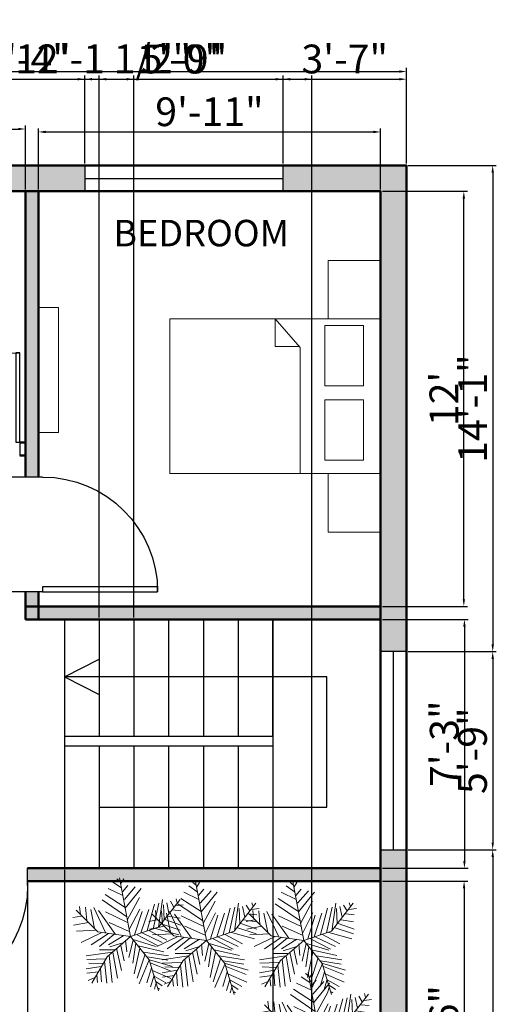
# Model space of a CAD drawing. Units: inches. Extents: x 1344 to 2521, y 3236 to 4924.
# Tile 7 of 14: x 2244 to 2410, y 3472 to 3814. Entities that reach past the tile are written whole.
import ezdxf

# ---------------------------------------------------------------- set-up
doc = ezdxf.new("R2010")
doc.units = ezdxf.units.IN
for name, color, linetype, lineweight in [('A-ANNO-DIMS', 2, 'Continuous', 18), ('A-AREA-IDEN', 3, 'Continuous', 18), ('A-DOOR', 50, 'Continuous', 25), ('A-FLOR-STRS', 7, 'Continuous', 25), ('A-FURN', 130, 'Continuous', 18), ('A-GLAZ', 150, 'Continuous', 25), ('A-WALL', 31, 'Continuous', 50), ('A-WALL-PATT', 8, 'Continuous', 13), ('L-PLNT', 82, 'Continuous', 13)]:
    doc.layers.add(name, color=color, linetype=linetype, lineweight=lineweight)
doc.styles.get("Standard").update_dxf_attribs({"font": 'arial.ttf'})
doc.dimstyles.new('ISO-25', dxfattribs={"dimtxt": 10, "dimasz": 2.5, "dimexe": 1.25, "dimexo": 0.625, "dimtad": 1, "dimdec": 0, "dimlunit": 4, "dimtxsty": 'Standard', "dimcen": 2.5, "dimadec": 0, "dimazin": 0, "dimtfac": 1, "dimtdec": 0, "dimtmove": 0, "dimatfit": 3, "dimfxl": 1, "dimarcsym": 0})

# ---------------------------------------------------------------- blocks, each defined once
blk = doc.blocks.new('*U2')
for p, q in [((0, 0), (0, -6)), ((40, 0), (40, -6))]:
    blk.add_line(p, q)
blk.add_lwpolyline([(0, 0), (0, 40), (1.75, 40), (1.75, 0)], close=True)
blk.add_arc((0, 0), 40, 0, 90)
blk = doc.blocks.new('*U8')
for p, q in [((-8.737, 47.138), (-17.069, 52.711)), ((-10.186, 53.64), (-13.084, 55.962)), ((0, 0), (-10.5, 57)), ((-9.099, 51.782), (-6.563, 55.962)), ((-7.65, 43.423), (-2.578, 49.46)), ((-5.839, 35.992), (4.667, 48.067)), ((-5.114, 28.097), (-24.676, 40.636)), ((-7.288, 39.707), (-21.778, 46.673)), ((-5.114, 27.632), (10.463, 46.673)), ((-48.585, 21.131), (-49.309, 29.026)), ((-3.665, 19.273), (-27.574, 35.527)), ((-2.941, 16.486), (8.652, 37.85)), ((16.259, 5.805), (23.142, 31.348)), ((22.055, 7.198), (27.489, 32.277)), ((27, 9), (48, 36)), ((27.127, 9.056), (31.112, 35.992)), ((31.836, 30.883), (32.561, 16.486)), ((35.096, 32.741), (37.27, 22.524)), ((38.719, 34.134), (41.979, 28.561)), ((43.791, 29.954), (51.036, 30.883)), ((44.153, 36.456), (45.239, 32.741)), ((-47.498, 19.737), (-55.83, 18.344)), ((-31.5, 4.5), (-52.5, 25.5)), ((-43.513, 28.561), (-42.427, 15.558)), ((-38.442, 26.239), (-34.819, 7.663)), ((-35.544, 28.097), (-24.314, 3.947)), ((-14.533, 2.09), (-30.834, 25.31)), ((-24.314, 23.917), (-2.941, 13.7)), ((-1.129, 6.734), (9.014, 26.704)), ((3.942, 1.625), (11.187, 24.381)), ((10.101, 3.483), (17.708, 26.239)), ((36.183, 19.737), (48.137, 17.88)), ((40.53, 25.775), (48.862, 24.846)), ((-40.615, 13.7), (-55.105, 10.913)), ((-20.691, 13.7), (-1.129, 4.876)), ((29.662, 12.307), (48.137, 6.269)), ((33.285, 16.486), (48.862, 10.913)), ((-33.37, 6.269), (-52.207, 5.34)), ((-28.299, 3.483), (-47.86, -5.805)), ((-21.416, 3.018), (-38.079, -8.128)), ((0, 0), (-31.5, 4.5)), ((-15.982, 2.09), (-30.11, -9.521)), ((0, 0), (-22.5, -19.5)), ((-6.563, 1.161), (-21.416, -8.128)), ((0, 0), (27, 9)), ((0, 0), (18, -22.5)), ((6.478, 1.625), (26.04, -8.592)), ((11.187, 3.483), (30.749, -5.805)), ((18.07, 5.805), (35.096, -3.483)), ((24.229, 7.663), (46.688, 1.625)), ((-6.563, -5.805), (-19.967, -9.985)), ((-9.461, -8.592), (-6.201, -23.453)), ((-4.752, -3.483), (-3.665, -14.629)), ((2.493, -3.019), (-1.491, -20.202)), ((1.769, -2.555), (24.229, -9.521)), ((5.029, -6.27), (2.131, -25.775)), ((7.565, -9.056), (32.198, -14.629)), ((-17.431, -15.094), (-42.789, -18.809)), ((-15.257, -12.772), (-30.11, -12.772)), ((-20.691, -18.345), (-17.793, -44.352)), ((-17.069, -15.094), (-12.721, -40.172)), ((-13.446, -11.378), (-8.737, -32.741)), ((9.014, -11.378), (3.58, -35.992)), ((14.085, -16.951), (6.478, -40.172)), ((12.274, -15.094), (36.907, -18.809)), ((-24.314, -21.596), (-42.427, -22.06)), ((-26.849, -26.24), (-40.253, -25.775)), ((-22.5, -19.5), (-37.5, -45)), ((-25.038, -23.918), (-22.865, -45.281)), ((18.07, -22.524), (8.289, -45.745)), ((16.259, -19.738), (36.183, -22.989)), ((18, -22.5), (27, -52.5)), ((18.433, -22.524), (40.53, -29.026)), ((19.157, -25.311), (38.719, -33.206)), ((-28.299, -29.026), (-42.789, -31.348)), ((-30.834, -34.135), (-42.427, -35.528)), ((-32.646, -36.921), (-31.921, -44.352)), ((-29.023, -30.884), (-27.936, -43.887)), ((20.244, -30.419), (15.897, -44.816)), ((22.78, -37.85), (19.519, -48.532)), ((21.331, -32.741), (39.081, -40.636)), ((-34.457, -39.708), (-40.978, -42.494)), ((22.78, -38.314), (34.372, -44.816)), ((24.591, -45.745), (23.142, -50.854)), ((24.591, -43.423), (30.749, -47.603)), ((26.764, -49.925), (28.213, -50.854))]:
    blk.add_line(p, q)
blk = doc.blocks.new('*D47')
at = {"layer": 'A-ANNO-DIMS', "color": 0, "lineweight": -2, "transparency": 16777216}
for p, q in [((2018.36, 3764.06), (2018.36, 3797.35)), ((2020.86, 3796.1), (2375.86, 3796.1)), ((2378.36, 3764.06), (2378.36, 3797.35))]:
    blk.add_line(p, q, dxfattribs=at)
at = {"layer": 'A-ANNO-DIMS', "color": 0, "lineweight": 100, "transparency": 16777216}
for points in [[(2020.86, 3796.52), (2020.86, 3795.69), (2018.36, 3796.1)], [(2375.86, 3796.52), (2375.86, 3795.69), (2378.36, 3796.1)]]:
    blk.add_solid(points, dxfattribs=at)
at = {"layer": 'Defpoints', "color": 0, "lineweight": 100, "transparency": 16777216}
for p in [(2378.36, 3796.1), (2018.36, 3763.43), (2378.36, 3763.43)]:
    blk.add_point(p, dxfattribs=at)
at = {"layer": 'A-ANNO-DIMS', "color": 0, "transparency": 16777216, "insert": (2198.36, 3801.84), "char_height": 10, "attachment_point": 5}
blk.add_mtext("30'", dxfattribs=at)
blk = doc.blocks.new('*D49')
at = {"layer": 'A-ANNO-DIMS', "color": 0, "lineweight": -2, "transparency": 16777216}
for p, q in [((2176.1, 3755.06), (2176.1, 3777.36)), ((2178.6, 3776.11), (2243.29, 3776.11)), ((2245.79, 3755.06), (2245.79, 3777.36))]:
    blk.add_line(p, q, dxfattribs=at)
at = {"layer": 'A-ANNO-DIMS', "color": 0, "lineweight": 100, "transparency": 16777216}
for points in [[(2178.6, 3776.53), (2178.6, 3775.69), (2176.1, 3776.11)], [(2243.29, 3776.53), (2243.29, 3775.69), (2245.79, 3776.11)]]:
    blk.add_solid(points, dxfattribs=at)
at = {"layer": 'Defpoints', "color": 0, "lineweight": 100, "transparency": 16777216}
for p in [(2245.79, 3776.11), (2176.1, 3754.43), (2245.79, 3754.43)]:
    blk.add_point(p, dxfattribs=at)
at = {"layer": 'A-ANNO-DIMS', "color": 0, "transparency": 16777216, "insert": (2210.94, 3781.84), "char_height": 10, "attachment_point": 5}
blk.add_mtext('5\'-10"', dxfattribs=at)
blk = doc.blocks.new('*D50')
at = {"layer": 'A-ANNO-DIMS', "color": 0, "lineweight": -2, "transparency": 16777216}
for p, q in [((2250.29, 3755.06), (2250.29, 3776.34)), ((2252.79, 3775.09), (2366.86, 3775.09)), ((2369.36, 3755.06), (2369.36, 3776.34))]:
    blk.add_line(p, q, dxfattribs=at)
at = {"layer": 'A-ANNO-DIMS', "color": 0, "lineweight": 100, "transparency": 16777216}
for points in [[(2252.79, 3775.5), (2252.79, 3774.67), (2250.29, 3775.09)], [(2366.86, 3775.5), (2366.86, 3774.67), (2369.36, 3775.09)]]:
    blk.add_solid(points, dxfattribs=at)
at = {"layer": 'Defpoints', "color": 0, "lineweight": 100, "transparency": 16777216}
for p in [(2369.36, 3775.09), (2250.29, 3754.43), (2369.36, 3754.43)]:
    blk.add_point(p, dxfattribs=at)
at = {"layer": 'A-ANNO-DIMS', "color": 0, "transparency": 16777216, "insert": (2309.83, 3780.82), "char_height": 10, "attachment_point": 5}
blk.add_mtext('9\'-11"', dxfattribs=at)
blk = doc.blocks.new('*D57')
at = {"layer": 'A-ANNO-DIMS', "color": 0, "lineweight": -2, "transparency": 16777216}
for p, q in [((2369.99, 3754.43), (2399.57, 3754.43)), ((2398.32, 3612.52), (2398.32, 3751.93)), ((2369.99, 3610.02), (2399.57, 3610.02))]:
    blk.add_line(p, q, dxfattribs=at)
at = {"layer": 'A-ANNO-DIMS', "color": 0, "lineweight": 100, "transparency": 16777216}
for points in [[(2397.9, 3751.93), (2398.73, 3751.93), (2398.32, 3754.43)], [(2397.9, 3612.52), (2398.73, 3612.52), (2398.32, 3610.02)]]:
    blk.add_solid(points, dxfattribs=at)
at = {"layer": 'Defpoints', "color": 0, "lineweight": 100, "transparency": 16777216}
for p in [(2369.36, 3754.43), (2398.32, 3754.43), (2369.36, 3610.02)]:
    blk.add_point(p, dxfattribs=at)
at = {"layer": 'A-ANNO-DIMS', "color": 0, "transparency": 16777216, "insert": (2392.67, 3682.23), "char_height": 10, "attachment_point": 5, "rotation": 90}
blk.add_mtext("12'", dxfattribs=at)
blk = doc.blocks.new('*D58')
at = {"layer": 'A-ANNO-DIMS', "color": 0, "lineweight": -2, "transparency": 16777216}
for p, q in [((2369.99, 3605.52), (2399.77, 3605.52)), ((2398.52, 3603.02), (2398.52, 3521.45)), ((2369.99, 3518.95), (2399.77, 3518.95))]:
    blk.add_line(p, q, dxfattribs=at)
at = {"layer": 'A-ANNO-DIMS', "color": 0, "lineweight": 100, "transparency": 16777216}
for points in [[(2398.11, 3603.02), (2398.94, 3603.02), (2398.52, 3605.52)], [(2398.11, 3521.45), (2398.94, 3521.45), (2398.52, 3518.95)]]:
    blk.add_solid(points, dxfattribs=at)
at = {"layer": 'Defpoints', "color": 0, "lineweight": 100, "transparency": 16777216}
for p in [(2369.36, 3605.52), (2369.36, 3518.95), (2398.52, 3518.95)]:
    blk.add_point(p, dxfattribs=at)
at = {"layer": 'A-ANNO-DIMS', "color": 0, "transparency": 16777216, "insert": (2392.79, 3562.24), "char_height": 10, "attachment_point": 5, "rotation": 90}
blk.add_mtext('7\'-3"', dxfattribs=at)
blk = doc.blocks.new('*D59')
at = {"layer": 'A-ANNO-DIMS', "color": 0, "lineweight": -2, "transparency": 16777216}
for p, q in [((2369.99, 3514.45), (2399.65, 3514.45)), ((2398.4, 3511.95), (2398.4, 3414.51)), ((2370.19, 3412.01), (2399.65, 3412.01))]:
    blk.add_line(p, q, dxfattribs=at)
at = {"layer": 'A-ANNO-DIMS', "color": 0, "lineweight": 100, "transparency": 16777216}
for points in [[(2397.98, 3511.95), (2398.82, 3511.95), (2398.4, 3514.45)], [(2397.98, 3414.51), (2398.82, 3414.51), (2398.4, 3412.01)]]:
    blk.add_solid(points, dxfattribs=at)
at = {"layer": 'Defpoints', "color": 0, "lineweight": 100, "transparency": 16777216}
for p in [(2369.36, 3514.45), (2369.57, 3412.01), (2398.4, 3412.01)]:
    blk.add_point(p, dxfattribs=at)
at = {"layer": 'A-ANNO-DIMS', "color": 0, "transparency": 16777216, "insert": (2392.67, 3463.23), "char_height": 10, "attachment_point": 5, "rotation": 90}
blk.add_mtext('8\'-6"', dxfattribs=at)
blk = doc.blocks.new('BED-DOUBLE')
for p, q in [((27.95, 53.78), (27.95, 9.98)), ((27.95, 9.98), (36.68, 0)), ((36.68, 9.56), (28.32, 9.56)), ((36.68, 0), (36.68, 9.56))]:
    blk.add_line(p, q)
for points in [[(0, 0), (73.35, 0), (73.35, 53.78), (0, 53.78)], [(5.91, 28.08), (19.39, 28.08), (19.39, 49.13), (5.91, 49.13)], [(5.91, 2.27), (19.39, 2.27), (19.39, 23.31), (5.91, 23.31)]]:
    blk.add_lwpolyline(points, close=True)
blk = doc.blocks.new('*D193')
at = {"layer": 'A-ANNO-DIMS', "color": 0, "lineweight": -2, "transparency": 16777216}
for p, q in [((2226.56, 3764.06), (2226.56, 3794.68)), ((2229.06, 3793.43), (2263.98, 3793.43)), ((2266.48, 3764.06), (2266.48, 3794.68))]:
    blk.add_line(p, q, dxfattribs=at)
at = {"layer": 'A-ANNO-DIMS', "color": 0, "lineweight": 100, "transparency": 16777216}
for points in [[(2229.06, 3793.85), (2229.06, 3793.02), (2226.56, 3793.43)], [(2263.98, 3793.85), (2263.98, 3793.02), (2266.48, 3793.43)]]:
    blk.add_solid(points, dxfattribs=at)
at = {"layer": 'Defpoints', "color": 0, "lineweight": 100, "transparency": 16777216}
for p in [(2266.48, 3793.43), (2226.56, 3763.43), (2266.48, 3763.43)]:
    blk.add_point(p, dxfattribs=at)
at = {"layer": 'A-ANNO-DIMS', "color": 0, "transparency": 16777216, "insert": (2246.52, 3799.17), "char_height": 10, "attachment_point": 5}
blk.add_mtext('3\'-4"', dxfattribs=at)
blk = doc.blocks.new('*D194')
at = {"layer": 'A-ANNO-DIMS', "color": 0, "lineweight": -2, "transparency": 16777216}
for p, q in [((2266.48, 3764.06), (2266.48, 3794.68)), ((2268.98, 3793.43), (2332.91, 3793.43)), ((2335.41, 3764.06), (2335.41, 3794.68))]:
    blk.add_line(p, q, dxfattribs=at)
at = {"layer": 'A-ANNO-DIMS', "color": 0, "lineweight": 100, "transparency": 16777216}
for points in [[(2268.98, 3793.85), (2268.98, 3793.02), (2266.48, 3793.43)], [(2332.91, 3793.85), (2332.91, 3793.02), (2335.41, 3793.43)]]:
    blk.add_solid(points, dxfattribs=at)
at = {"layer": 'Defpoints', "color": 0, "lineweight": 100, "transparency": 16777216}
for p in [(2335.41, 3793.43), (2266.48, 3763.43), (2335.41, 3763.43)]:
    blk.add_point(p, dxfattribs=at)
at = {"layer": 'A-ANNO-DIMS', "color": 0, "transparency": 16777216, "insert": (2300.95, 3799.16), "char_height": 10, "attachment_point": 5}
blk.add_mtext('5\'-9"', dxfattribs=at)
blk = doc.blocks.new('*D195')
at = {"layer": 'A-ANNO-DIMS', "color": 0, "lineweight": -2, "transparency": 16777216}
for p, q in [((2335.41, 3764.06), (2335.41, 3794.68)), ((2337.91, 3793.43), (2375.86, 3793.43)), ((2378.36, 3764.06), (2378.36, 3794.68))]:
    blk.add_line(p, q, dxfattribs=at)
at = {"layer": 'A-ANNO-DIMS', "color": 0, "lineweight": 100, "transparency": 16777216}
for points in [[(2337.91, 3793.85), (2337.91, 3793.02), (2335.41, 3793.43)], [(2375.86, 3793.85), (2375.86, 3793.02), (2378.36, 3793.43)]]:
    blk.add_solid(points, dxfattribs=at)
at = {"layer": 'Defpoints', "color": 0, "lineweight": 100, "transparency": 16777216}
for p in [(2378.36, 3793.43), (2335.41, 3763.43), (2378.36, 3763.43)]:
    blk.add_point(p, dxfattribs=at)
at = {"layer": 'A-ANNO-DIMS', "color": 0, "transparency": 16777216, "insert": (2356.89, 3799.17), "char_height": 10, "attachment_point": 5}
blk.add_mtext('3\'-7"', dxfattribs=at)
blk = doc.blocks.new('*D203')
at = {"layer": 'A-ANNO-DIMS', "color": 0, "lineweight": -2, "transparency": 16777216}
for p, q in [((2378.99, 3763.43), (2409.61, 3763.43)), ((2408.36, 3760.93), (2408.36, 3596.78)), ((2378.99, 3594.28), (2409.61, 3594.28))]:
    blk.add_line(p, q, dxfattribs=at)
at = {"layer": 'A-ANNO-DIMS', "color": 0, "lineweight": 100, "transparency": 16777216}
for points in [[(2407.95, 3760.93), (2408.78, 3760.93), (2408.36, 3763.43)], [(2407.95, 3596.78), (2408.78, 3596.78), (2408.36, 3594.28)]]:
    blk.add_solid(points, dxfattribs=at)
at = {"layer": 'Defpoints', "color": 0, "lineweight": 100, "transparency": 16777216}
for p in [(2378.36, 3763.43), (2378.36, 3594.28), (2408.36, 3594.28)]:
    blk.add_point(p, dxfattribs=at)
at = {"layer": 'A-ANNO-DIMS', "color": 0, "transparency": 16777216, "insert": (2402.72, 3678.86), "char_height": 10, "attachment_point": 5, "rotation": 90}
blk.add_mtext('14\'-1"', dxfattribs=at)
blk = doc.blocks.new('*D204')
at = {"layer": 'A-ANNO-DIMS', "color": 0, "lineweight": -2, "transparency": 16777216}
for p, q in [((2378.99, 3594.28), (2409.61, 3594.28)), ((2408.36, 3591.78), (2408.36, 3527.86)), ((2378.99, 3525.36), (2409.61, 3525.36))]:
    blk.add_line(p, q, dxfattribs=at)
at = {"layer": 'A-ANNO-DIMS', "color": 0, "lineweight": 100, "transparency": 16777216}
for points in [[(2407.95, 3591.78), (2408.78, 3591.78), (2408.36, 3594.28)], [(2407.95, 3527.86), (2408.78, 3527.86), (2408.36, 3525.36)]]:
    blk.add_solid(points, dxfattribs=at)
at = {"layer": 'Defpoints', "color": 0, "lineweight": 100, "transparency": 16777216}
for p in [(2378.36, 3594.28), (2378.36, 3525.36), (2408.36, 3525.36)]:
    blk.add_point(p, dxfattribs=at)
at = {"layer": 'A-ANNO-DIMS', "color": 0, "transparency": 16777216, "insert": (2402.63, 3559.82), "char_height": 10, "attachment_point": 5, "rotation": 90}
blk.add_mtext('5\'-9"', dxfattribs=at)
blk = doc.blocks.new('*D205')
at = {"layer": 'A-ANNO-DIMS', "color": 0, "lineweight": -2, "transparency": 16777216}
for p, q in [((2378.99, 3525.36), (2409.61, 3525.36)), ((2408.36, 3522.86), (2408.36, 3350.01)), ((2378.99, 3347.51), (2409.61, 3347.51))]:
    blk.add_line(p, q, dxfattribs=at)
at = {"layer": 'A-ANNO-DIMS', "color": 0, "lineweight": 100, "transparency": 16777216}
for points in [[(2407.95, 3522.86), (2408.78, 3522.86), (2408.36, 3525.36)], [(2407.95, 3350.01), (2408.78, 3350.01), (2408.36, 3347.51)]]:
    blk.add_solid(points, dxfattribs=at)
at = {"layer": 'Defpoints', "color": 0, "lineweight": 100, "transparency": 16777216}
for p in [(2378.36, 3525.36), (2378.36, 3347.51), (2408.36, 3347.51)]:
    blk.add_point(p, dxfattribs=at)
at = {"layer": 'A-ANNO-DIMS', "color": 0, "transparency": 16777216, "insert": (2402.63, 3436.44), "char_height": 10, "attachment_point": 5, "rotation": 90}
blk.add_mtext('14\'-10"', dxfattribs=at)
blk = doc.blocks.new('*D214')
at = {"layer": 'A-ANNO-DIMS', "color": 0, "lineweight": -2, "transparency": 16777216}
for p, q in [((2249.66, 3655.04), (1987.11, 3655.04)), ((1988.36, 3652.54), (1988.36, 3617.54)), ((2249.66, 3615.04), (1987.11, 3615.04))]:
    blk.add_line(p, q, dxfattribs=at)
at = {"layer": 'A-ANNO-DIMS', "color": 0, "lineweight": 100, "transparency": 16777216}
for points in [[(1987.95, 3652.54), (1988.78, 3652.54), (1988.36, 3655.04)], [(1987.95, 3617.54), (1988.78, 3617.54), (1988.36, 3615.04)]]:
    blk.add_solid(points, dxfattribs=at)
at = {"layer": 'Defpoints', "color": 0, "lineweight": 100, "transparency": 16777216}
for p in [(2250.29, 3655.04), (1988.36, 3615.04), (2250.29, 3615.04)]:
    blk.add_point(p, dxfattribs=at)
at = {"layer": 'A-ANNO-DIMS', "color": 0, "transparency": 16777216, "insert": (1982.63, 3635.04), "char_height": 10, "attachment_point": 5, "rotation": 90}
blk.add_mtext('3\'-4"', dxfattribs=at)
blk = doc.blocks.new('*D215')
at = {"layer": 'A-ANNO-DIMS', "color": 0, "lineweight": -2, "transparency": 16777216}
for p, q in [((2206.56, 3513.82), (2206.56, 3316.22)), ((2246.56, 3513.82), (2246.56, 3316.22)), ((2209.06, 3317.47), (2244.06, 3317.47))]:
    blk.add_line(p, q, dxfattribs=at)
at = {"layer": 'A-ANNO-DIMS', "color": 0, "lineweight": 100, "transparency": 16777216}
for points in [[(2209.06, 3317.89), (2209.06, 3317.06), (2206.56, 3317.47)], [(2244.06, 3317.89), (2244.06, 3317.06), (2246.56, 3317.47)]]:
    blk.add_solid(points, dxfattribs=at)
at = {"layer": 'Defpoints', "color": 0, "lineweight": 100, "transparency": 16777216}
for p in [(2206.56, 3514.45), (2246.56, 3514.45), (2246.56, 3317.47)]:
    blk.add_point(p, dxfattribs=at)
at = {"layer": 'A-ANNO-DIMS', "color": 0, "transparency": 16777216, "insert": (2226.56, 3323.21), "char_height": 10, "attachment_point": 5}
blk.add_mtext('3\'-4"', dxfattribs=at)
blk = doc.blocks.new('*D217')
at = {"layer": 'A-ANNO-DIMS', "color": 0, "lineweight": -2, "transparency": 16777216}
for p, q in [((2200.2, 3403.64), (2200.2, 3794.68)), ((2202.7, 3793.43), (2342.96, 3793.43)), ((2345.46, 3403.64), (2345.46, 3794.68))]:
    blk.add_line(p, q, dxfattribs=at)
at = {"layer": 'A-ANNO-DIMS', "color": 0, "lineweight": 100, "transparency": 16777216}
for points in [[(2202.7, 3793.85), (2202.7, 3793.02), (2200.2, 3793.43)], [(2342.96, 3793.85), (2342.96, 3793.02), (2345.46, 3793.43)]]:
    blk.add_solid(points, dxfattribs=at)
at = {"layer": 'Defpoints', "color": 0, "lineweight": 100, "transparency": 16777216}
for p in [(2345.46, 3793.43), (2200.2, 3403.01), (2345.46, 3403.01)]:
    blk.add_point(p, dxfattribs=at)
at = {"layer": 'A-ANNO-DIMS', "color": 0, "transparency": 16777216, "insert": (2272.83, 3799.23), "char_height": 10, "attachment_point": 5}
blk.add_mtext('12\'-1 1/2"', dxfattribs=at)
blk = doc.blocks.new('*D218')
at = {"layer": 'A-ANNO-DIMS', "color": 0, "lineweight": -2, "transparency": 16777216}
for p, q in [((2259.38, 3518.32), (2259.38, 3316.22)), ((2331.86, 3518.32), (2331.86, 3316.22)), ((2261.88, 3317.47), (2329.36, 3317.47))]:
    blk.add_line(p, q, dxfattribs=at)
at = {"layer": 'A-ANNO-DIMS', "color": 0, "lineweight": 100, "transparency": 16777216}
for points in [[(2261.88, 3317.89), (2261.88, 3317.06), (2259.38, 3317.47)], [(2329.36, 3317.89), (2329.36, 3317.06), (2331.86, 3317.47)]]:
    blk.add_solid(points, dxfattribs=at)
at = {"layer": 'Defpoints', "color": 0, "lineweight": 100, "transparency": 16777216}
for p in [(2259.38, 3518.95), (2331.86, 3518.95), (2331.86, 3317.47)]:
    blk.add_point(p, dxfattribs=at)
at = {"layer": 'A-ANNO-DIMS', "color": 0, "transparency": 16777216, "insert": (2295.62, 3323.27), "char_height": 10, "attachment_point": 5}
blk.add_mtext('6\'-0 1/2"', dxfattribs=at)
blk = doc.blocks.new('*D219')
at = {"layer": 'A-ANNO-DIMS', "color": 0, "lineweight": -2, "transparency": 16777216}
for p, q in [((2271.46, 3606.15), (2271.46, 3794.68)), ((2273.96, 3793.43), (2281.04, 3793.43)), ((2283.54, 3606.15), (2283.54, 3794.68)), ((2283.54, 3793.43), (2312.93, 3793.43))]:
    blk.add_line(p, q, dxfattribs=at)
at = {"layer": 'A-ANNO-DIMS', "color": 0, "lineweight": 100, "transparency": 16777216}
for points in [[(2273.96, 3793.85), (2273.96, 3793.02), (2271.46, 3793.43)], [(2281.04, 3793.85), (2281.04, 3793.02), (2283.54, 3793.43)]]:
    blk.add_solid(points, dxfattribs=at)
at = {"layer": 'Defpoints', "color": 0, "lineweight": 100, "transparency": 16777216}
for p in [(2283.54, 3793.43), (2271.46, 3605.52), (2283.54, 3605.52)]:
    blk.add_point(p, dxfattribs=at)
at = {"layer": 'A-ANNO-DIMS', "color": 0, "transparency": 16777216, "insert": (2299.49, 3799.16), "char_height": 10, "attachment_point": 5}
blk.add_mtext('1\'-0"', dxfattribs=at)

msp = doc.modelspace()

# ---------------------------------------------------------------- hatches: boundary and pattern name
at = {"layer": 'A-WALL-PATT'}
h = msp.add_hatch(color=256, dxfattribs=at)
h.dxf.hatch_style = 1
h.paths.add_polyline_path([(2193.45, 3763.43), (2126.57, 3763.43), (2126.57, 3754.43), (2193.45, 3754.43)])
h.paths.add_polyline_path([(2057.65, 3763.43), (2018.36, 3763.43), (2018.36, 3608.87), (2027.36, 3608.87), (2027.36, 3754.43), (2057.65, 3754.43)])
h.paths.add_polyline_path([(2266.48, 3763.43), (2226.56, 3763.43), (2226.56, 3754.43), (2266.48, 3754.43)])
h.paths.add_polyline_path([(2378.36, 3763.43), (2335.41, 3763.43), (2335.41, 3754.43), (2369.36, 3754.43), (2369.36, 3594.28), (2378.36, 3594.28)])
h.paths.add_polyline_path([(2369.36, 3610.02), (2250.29, 3610.02), (2250.29, 3605.52), (2369.36, 3605.52)])
h.paths.add_polyline_path([(2250.29, 3610.02), (2245.79, 3610.02), (2245.79, 3605.52), (2250.29, 3605.52)])
h.paths.add_polyline_path([(2250.29, 3754.43), (2245.79, 3754.43), (2245.79, 3655.04), (2250.29, 3655.04)])
h.paths.add_polyline_path([(2176.1, 3754.43), (2171.6, 3754.43), (2171.6, 3624.19), (2171.35, 3624.19), (2169.02, 3624.19), (2169.02, 3619.69), (2176.1, 3619.69)])
h.paths.add_polyline_path([(2129.02, 3624.19), (2122.52, 3624.19), (2122.52, 3619.69), (2129.02, 3619.69)])
h.paths.add_polyline_path([(2091.69, 3624.19), (2027.36, 3624.19), (2027.36, 3619.69), (2091.72, 3619.69, -0.012876), (2091.69, 3620.84)])
h.paths.add_polyline_path([(2250.29, 3615.04), (2245.79, 3615.04), (2245.79, 3610.02), (2250.29, 3610.02)])
h.paths.add_polyline_path([(2027.36, 3580.89), (2018.36, 3580.89), (2018.36, 3555.45), (2027.36, 3555.45)])
h.paths.add_polyline_path([(2027.36, 3527.47), (2018.36, 3527.47), (2018.36, 3455.82), (2027.36, 3455.82)])
h.paths.add_polyline_path([(2093.06, 3517.8, -0.012876), (2093.09, 3518.95), (2027.36, 3518.95), (2027.36, 3514.45), (2093.06, 3514.45)])
h.paths.add_polyline_path([(2118.02, 3573.32), (2110.02, 3573.32), (2110.02, 3573.28), (2080.51, 3573.28), (2027.36, 3573.32), (2027.36, 3568.82), (2118.02, 3568.82)])
h.paths.add_polyline_path([(2122.52, 3624.19), (2114.02, 3624.19), (2114.02, 3620.84), (2114.02, 3619.69), (2118.02, 3619.69), (2118.02, 3518.95), (2122.52, 3518.95)])
h.paths.add_polyline_path([(2129.02, 3518.95), (2115.39, 3518.95), (2115.39, 3517.8), (2115.39, 3514.45), (2129.02, 3514.45)])
h.paths.add_polyline_path([(2027.36, 3386.9), (2018.36, 3386.9), (2018.36, 3347.51), (2056.7, 3347.51), (2056.7, 3356.47), (2027.36, 3356.47)])
h.paths.add_polyline_path([(2187.76, 3356.47), (2168.81, 3356.47), (2149.67, 3356.47), (2125.62, 3356.47), (2125.62, 3347.51), (2176.1, 3347.51), (2187.76, 3347.51)])
h.paths.add_polyline_path([(2378.36, 3525.36), (2369.36, 3525.36), (2369.36, 3497.27), (2369.36, 3412.01), (2369.57, 3412.01), (2369.57, 3403.01), (2369.36, 3356.51), (2369.36, 3347.51), (2378.36, 3347.51)])
h.paths.add_polyline_path([(2369.36, 3412.01), (2345.46, 3412.01), (2345.46, 3403.01), (2369.36, 3403.01)])
h.paths.add_polyline_path([(2206.56, 3518.95), (2176.1, 3518.95), (2176.1, 3514.45), (2206.56, 3514.45)])
h.paths.add_polyline_path([(2130.92, 3560.64), (2239.92, 3560.64), (2239.92, 3579.62), (2130.92, 3579.62)], flags=9)
h.paths.add_polyline_path([(2271.24, 3730.09), (2345.91, 3730.09), (2345.91, 3749.07), (2271.24, 3749.07)], flags=9)
h.paths.add_polyline_path([(2051.28, 3467.76), (2122.39, 3467.76), (2122.39, 3502.26), (2051.28, 3502.26)], flags=9)
h.paths.add_polyline_path([(2033.92, 3520.24), (2083.56, 3520.24), (2083.56, 3539.22), (2033.92, 3539.22)], flags=9)
h.paths.add_polyline_path([(2030.69, 3603.57), (2080.34, 3603.57), (2080.34, 3622.55), (2030.69, 3622.55)], flags=9)
h.paths.add_polyline_path([(2175.78, 3699.42), (2225.43, 3699.42), (2225.43, 3718.41), (2175.78, 3718.41)], flags=9)
h.paths.add_polyline_path([(2051.88, 3718.72), (2122.99, 3718.72), (2122.99, 3753.22), (2051.88, 3753.22)], flags=9)
h = msp.add_hatch(color=256, dxfattribs=at)
h.dxf.hatch_style = 1
h.paths.add_polyline_path([(2200.2, 3412.01), (2176.1, 3412.01), (2176.1, 3403.01), (2200.2, 3403.01)])
h.paths.add_polyline_path([(2369.36, 3518.95), (2246.56, 3518.95), (2246.56, 3514.45), (2369.36, 3514.45)])
h.paths.add_polyline_path([(2130.92, 3560.64), (2239.92, 3560.64), (2239.92, 3579.62), (2130.92, 3579.62)], flags=9)
h.paths.add_polyline_path([(2271.24, 3730.09), (2345.91, 3730.09), (2345.91, 3749.07), (2271.24, 3749.07)], flags=9)
h.paths.add_polyline_path([(2051.28, 3467.76), (2122.39, 3467.76), (2122.39, 3502.26), (2051.28, 3502.26)], flags=9)
h.paths.add_polyline_path([(2033.92, 3520.24), (2083.56, 3520.24), (2083.56, 3539.22), (2033.92, 3539.22)], flags=9)
h.paths.add_polyline_path([(2030.69, 3603.57), (2080.34, 3603.57), (2080.34, 3622.55), (2030.69, 3622.55)], flags=9)
h.paths.add_polyline_path([(2175.78, 3699.42), (2225.43, 3699.42), (2225.43, 3718.41), (2175.78, 3718.41)], flags=9)
h.paths.add_polyline_path([(2051.88, 3718.72), (2122.99, 3718.72), (2122.99, 3753.22), (2051.88, 3753.22)], flags=9)

# ---------------------------------------------------------------- linework, layer by layer
at = {"layer": 'A-FLOR-STRS'}
for p, q in [((2259.38, 3605.52), (2259.38, 3518.95)), ((2271.46, 3605.52), (2271.46, 3564.91)), ((2283.54, 3605.52), (2283.54, 3564.91)), ((2295.62, 3605.52), (2295.62, 3564.91)), ((2307.7, 3605.52), (2307.7, 3564.91)), ((2319.78, 3605.52), (2319.78, 3564.91)), ((2331.86, 3564.91), (2331.86, 3605.52)), ((2331.86, 3605.52), (2331.86, 3518.95)), ((2259.38, 3585.5), (2271.46, 3591.67)), ((2350.63, 3585.5), (2259.38, 3585.5)), ((2259.38, 3585.5), (2271.46, 3579.32)), ((2350.63, 3540.2), (2350.63, 3585.5)), ((2271.46, 3561.45), (2271.46, 3518.95)), ((2283.54, 3561.45), (2283.54, 3518.95)), ((2295.62, 3561.45), (2295.62, 3518.95)), ((2307.7, 3561.45), (2307.7, 3518.95)), ((2319.78, 3561.45), (2319.78, 3518.95)), ((2271.46, 3540.2), (2350.63, 3540.2))]:
    msp.add_line(p, q, dxfattribs=at)
msp.add_lwpolyline([(2259.38, 3564.91), (2331.86, 3564.91), (2331.86, 3561.45), (2259.38, 3561.45)], dxfattribs=at)
at = {"layer": 'A-FURN'}
for points in [[(2369.36, 3730.36), (2351.14, 3730.36), (2351.14, 3710.02), (2369.36, 3710.02)], [(2250.29, 3670.57), (2257.27, 3670.57), (2257.27, 3714.04), (2250.29, 3714.04)], [(2369.36, 3656.24), (2351.14, 3656.24), (2351.14, 3635.89), (2369.36, 3635.89)]]:
    msp.add_lwpolyline(points, close=True, dxfattribs=at)
at = {"layer": 'A-GLAZ'}
for p, q in [((2266.48, 3758.93), (2335.41, 3758.93)), ((2373.86, 3525.36), (2373.86, 3594.28))]:
    msp.add_line(p, q, dxfattribs=at)
for points in [[(2266.48, 3763.43), (2266.48, 3754.43), (2335.41, 3754.43), (2335.41, 3763.43)], [(2369.36, 3525.36), (2378.36, 3525.36), (2378.36, 3594.28), (2369.36, 3594.28)]]:
    msp.add_lwpolyline(points, close=True, dxfattribs=at)
at = {"layer": 'A-WALL'}
for p, q in [((2245.79, 3655.04), (2245.79, 3754.43)), ((2250.29, 3655.04), (2250.29, 3754.43)), ((2245.79, 3735.69), (2245.79, 3655.04)), ((2250.29, 3735.69), (2250.29, 3655.04)), ((2243.8, 3666.99), (2245.79, 3666.99)), ((2243.8, 3662.49), (2245.79, 3662.49)), ((2245.79, 3615.04), (2245.79, 3605.52)), ((2245.79, 3605.52), (2245.79, 3615.04)), ((2250.29, 3615.04), (2250.29, 3605.52)), ((2250.29, 3605.52), (2250.29, 3615.04)), ((2369.36, 3610.02), (2245.79, 3610.02)), ((2369.36, 3605.52), (2245.79, 3605.52)), ((2369.36, 3533.27), (2369.36, 3497.27)), ((2246.56, 3518.95), (2369.36, 3518.95)), ((2246.56, 3518.95), (2248.05, 3518.95)), ((2246.56, 3514.45), (2369.36, 3514.45)), ((2246.56, 3514.45), (2261.58, 3514.45))]:
    msp.add_line(p, q, dxfattribs=at)
for points in [[(2378.36, 3347.51), (2378.36, 3763.43), (2018.36, 3763.43), (2018.36, 3347.51)], [(2369.36, 3356.51), (2369.36, 3754.43), (2027.36, 3754.43), (2027.36, 3356.47)]]:
    msp.add_lwpolyline(points, dxfattribs=at)

# ---------------------------------------------------------------- block references
at = {"layer": 'A-DOOR', "xscale": -0.7782718260199863, "yscale": 0.7782718260199863, "zscale": 0.7782718260199863}
msp.add_blockref('*U2', (2243.8, 3667.16), dxfattribs=at)
at = {"layer": 'A-DOOR', "xscale": -1}
for p, rotation in [((2251.79, 3615.04), 270), ((2206.56, 3512.95), 180)]:
    msp.add_blockref('*U2', p, dxfattribs=dict(at, rotation=rotation))
at = {"layer": 'A-FURN', "rotation": 180}
msp.add_blockref('BED-DOUBLE', (2369.36, 3710.02), dxfattribs=at)
at = {"layer": 'L-PLNT', "xscale": 0.3591539065448135, "yscale": 0.3591539065448135, "zscale": 0.3591539065448135}
for p in [(2282.35, 3495.16), (2308.74, 3493.84), (2342.6, 3493.84), (2347.88, 3462.21)]:
    msp.add_blockref('*U8', p, dxfattribs=at)

# ---------------------------------------------------------------- texts
at = {"layer": 'A-AREA-IDEN', "insert": (2273.54, 3744.5), "char_height": 9.211, "attachment_point": 1}
msp.add_mtext_dynamic_manual_height_columns(' BEDROOM', width=108.7809, gutter_width=46.06, heights=[0], dxfattribs=at)

# ---------------------------------------------------------------- dimensions: what is measured, and where the dimension line sits
at = {"layer": 'A-ANNO-DIMS'}
for base, p1, p2, override, picture, middle in [((2345.46, 3793.43), (2200.2, 3403.01), (2345.46, 3403.01), {"dimdec": 1, "dimlfac": 1, "dimrnd": 0, "dimzin": 1, "dimdsep": 46, "dimlunit": 4, "dimfrac": 2}, '*D217', (2272.83, 3799.23)), ((2378.36, 3796.1), (2018.36, 3763.43), (2378.36, 3763.43), {"dimclrd": 0, "dimclre": 0, "dimclrt": 0}, '*D47', (2198.36, 3801.84)), ((2266.48, 3793.43), (2226.56, 3763.43), (2266.48, 3763.43), {"dimdec": 1, "dimlfac": 1, "dimrnd": 0, "dimzin": 1, "dimdsep": 46, "dimlunit": 4, "dimfrac": 2}, '*D193', (2246.52, 3799.17)), ((2335.41, 3793.43), (2266.48, 3763.43), (2335.41, 3763.43), {"dimdec": 1, "dimlfac": 1, "dimrnd": 0, "dimzin": 1, "dimdsep": 46, "dimlunit": 4, "dimfrac": 2}, '*D194', (2300.95, 3799.16)), ((2283.54, 3793.43), (2271.46, 3605.52), (2283.54, 3605.52), {"dimdec": 1, "dimlfac": 1, "dimrnd": 0, "dimzin": 1, "dimdsep": 46, "dimlunit": 4, "dimfrac": 2}, '*D219', (2299.49, 3799.16)), ((2378.3631, 3793.4321), (2335.4077, 3763.4321), (2378.3631, 3763.4321), {"dimdec": 1, "dimlfac": 1, "dimrnd": 0, "dimzin": 1, "dimdsep": 46, "dimlunit": 4, "dimfrac": 2}, '*D195', (2356.8854, 3799.1662)), ((2245.79, 3776.11), (2176.1, 3754.43), (2245.79, 3754.43), {"dimclrd": 0, "dimclre": 0, "dimclrt": 0}, '*D49', (2210.94, 3781.84)), ((2369.36, 3775.09), (2250.29, 3754.43), (2369.36, 3754.43), {"dimclrd": 0, "dimclre": 0, "dimclrt": 0}, '*D50', (2309.83, 3780.82)), ((2331.86, 3317.47), (2259.38, 3518.95), (2331.86, 3518.95), {"dimdec": 1, "dimlfac": 1, "dimrnd": 0, "dimzin": 1, "dimdsep": 46, "dimlunit": 4, "dimfrac": 2}, '*D218', (2295.62, 3323.27)), ((2246.56, 3317.47), (2206.56, 3514.45), (2246.56, 3514.45), {"dimdec": 1, "dimlfac": 1, "dimrnd": 0, "dimzin": 1, "dimdsep": 46, "dimlunit": 4, "dimfrac": 2}, '*D215', (2226.56, 3323.21))]:
    dim = msp.add_linear_dim(base=base, p1=p1, p2=p2, dimstyle='ISO-25', override=override, dxfattribs=at)
    dim.commit()
    dim.dimension.update_dxf_attribs({"geometry": picture, "text_midpoint": middle})
for base, p1, p2, override, picture, middle in [((2408.3631, 3594.2838), (2378.3631, 3763.4321), (2378.3631, 3594.2838), {"dimdec": 1, "dimlfac": 1, "dimrnd": 0, "dimzin": 1, "dimdsep": 46, "dimlunit": 4, "dimfrac": 2}, '*D203', (2402.7177, 3678.858)), ((2398.32, 3754.43), (2369.36, 3610.02), (2369.36, 3754.43), {"dimclrd": 0, "dimclre": 0, "dimclrt": 0}, '*D57', (2392.67, 3682.23)), ((1988.36, 3615.04), (2250.29, 3655.04), (2250.29, 3615.04), {"dimdec": 1, "dimlfac": 1, "dimrnd": 0, "dimzin": 1, "dimdsep": 46, "dimlunit": 4, "dimfrac": 2}, '*D214', (1982.63, 3635.04)), ((2398.52, 3518.95), (2369.36, 3605.52), (2369.36, 3518.95), {"dimclrd": 0, "dimclre": 0, "dimclrt": 0}, '*D58', (2392.79, 3562.24)), ((2408.36, 3525.36), (2378.36, 3594.28), (2378.36, 3525.36), {"dimdec": 1, "dimlfac": 1, "dimrnd": 0, "dimzin": 1, "dimdsep": 46, "dimlunit": 4, "dimfrac": 2}, '*D204', (2402.63, 3559.82)), ((2408.3631, 3347.5114), (2378.3631, 3525.3602), (2378.3631, 3347.5114), {"dimdec": 1, "dimlfac": 1, "dimrnd": 0, "dimzin": 1, "dimdsep": 46, "dimlunit": 4, "dimfrac": 2}, '*D205', (2402.6324, 3436.4358)), ((2398.4, 3412.01), (2369.36, 3514.45), (2369.57, 3412.01), {"dimclrd": 0, "dimclre": 0, "dimclrt": 0}, '*D59', (2392.67, 3463.23))]:
    dim = msp.add_linear_dim(base=base, p1=p1, p2=p2, angle=90, dimstyle='ISO-25', override=override, dxfattribs=at)
    dim.commit()
    dim.dimension.update_dxf_attribs({"geometry": picture, "text_midpoint": middle})

doc.saveas('drawing.dxf')
